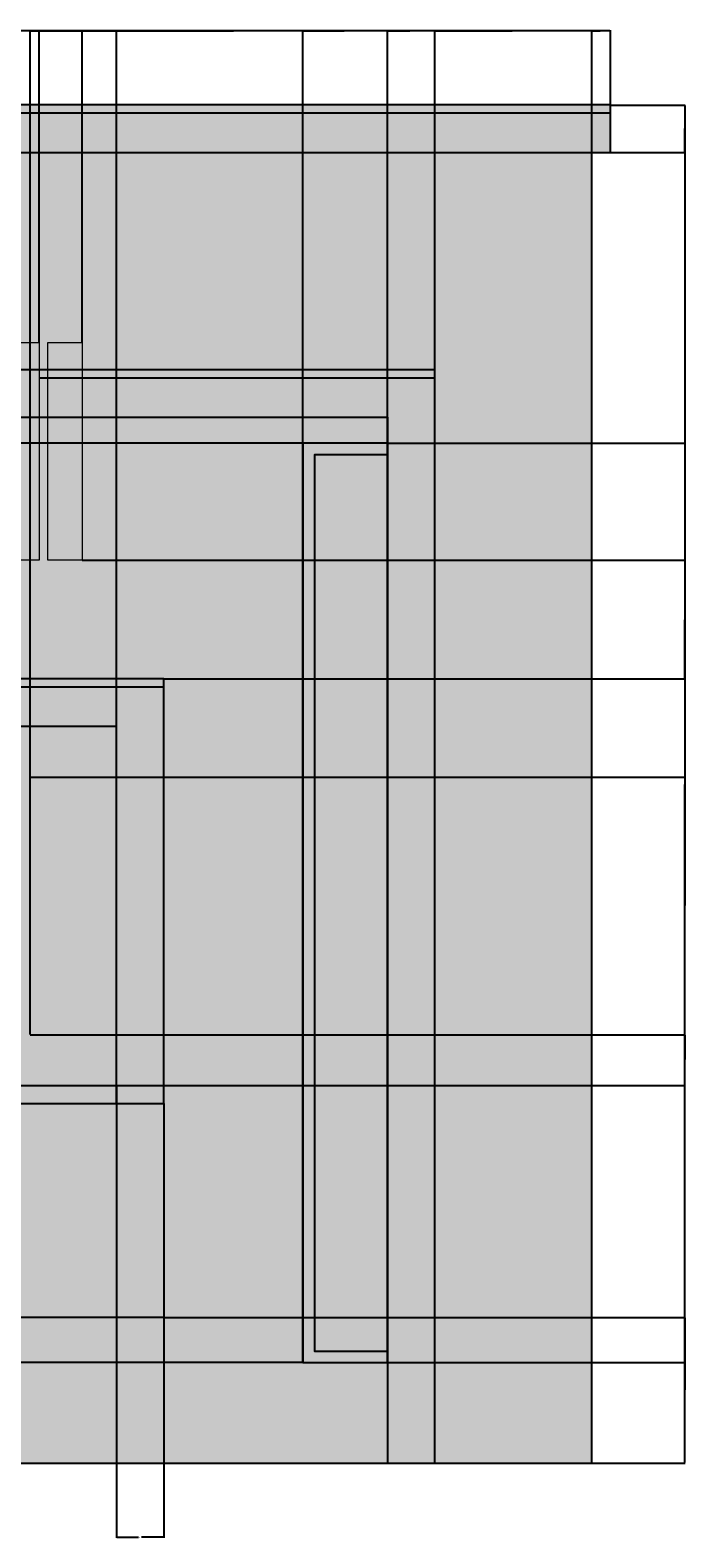
# Model space of a CAD drawing. Units: feet. Extents: x 2926 to 4178, y 965 to 1469.
# Tile 6 of 9: x 3245 to 3464, y 965 to 1469. Entities that reach past the tile are written whole.
import ezdxf

# ---------------------------------------------------------------- set-up
doc = ezdxf.new("R2010")
doc.units = ezdxf.units.FT
for name, color, linetype, lineweight in [('A-ANNO-DIMS', 2, 'Continuous', 18), ('A-ELEV', 7, 'Continuous', 25), ('A-ELEV-DETL', 8, 'Continuous', 18), ('A-ELEV-PATT', 9, 'Continuous', 13)]:
    doc.layers.add(name, color=color, linetype=linetype, lineweight=lineweight)
doc.styles.get("Standard").update_dxf_attribs({"font": 'arial.ttf'})
doc.dimstyles.get("Standard").update_dxf_attribs({"dimtxt": 0.18, "dimasz": 0.18, "dimexe": 0.18, "dimexo": 0.0625, "dimgap": 0.09, "dimtad": 0, "dimtih": 1, "dimtoh": 1, "dimdec": 1, "dimzin": 0, "dimdsep": 46, "dimlunit": 3, "dimtxsty": 'Standard', "dimcen": 0.09, "dimadec": 0, "dimazin": 0, "dimtfac": 1, "dimtdec": 1, "dimtofl": 0, "dimtmove": 0, "dimatfit": 3, "dimfxl": 1, "dimtolj": 1, "dimtzin": 0, "dimarcsym": 0})

# ---------------------------------------------------------------- blocks, each defined once
blk = doc.blocks.new('FACADE-FIN')
blk.add_lwpolyline([(0, 72.66), (11.46, 72.66), (11.46, 0), (0, 0)], close=True)
blk.add_lwpolyline([(0, 72.66), (11.46, 72.66), (11.46, 0), (0, 0)], close=True)
blk = doc.blocks.new('*D10')
at = {"layer": 'A-ANNO-DIMS', "color": 0, "lineweight": -2, "transparency": 16777216}
for p, q in [((2952.4, 1298.4), (2952.4, 1468.62)), ((2952.58, 1468.44), (3195.09, 1468.44)), ((3438.39, 1468.44), (3195.88, 1468.44)), ((3438.57, 1443.71), (3438.57, 1468.62))]:
    blk.add_line(p, q, dxfattribs=at)
at = {"layer": 'A-ANNO-DIMS', "color": 0, "transparency": 16777216}
for points in [[(2952.58, 1468.47), (2952.58, 1468.41), (2952.4, 1468.44)], [(3438.39, 1468.47), (3438.39, 1468.41), (3438.57, 1468.44)]]:
    blk.add_solid(points, dxfattribs=at)
at = {"layer": 'Defpoints', "color": 0, "transparency": 16777216}
for p in [(3438.57, 1468.44), (3438.57, 1443.64), (2952.4, 1298.33)]:
    blk.add_point(p, dxfattribs=at)
at = {"layer": 'A-ANNO-DIMS', "color": 0, "transparency": 16777216, "insert": (3195.49, 1468.44), "char_height": 0.18, "attachment_point": 5}
blk.add_mtext('\\A1;486.2', dxfattribs=at)
blk = doc.blocks.new('*D11')
at = {"layer": 'A-ANNO-DIMS', "color": 0, "lineweight": -2, "transparency": 16777216}
for p, q in [((3438.63, 1443.64), (3463.55, 1443.64)), ((3463.37, 1443.46), (3463.37, 1217.17)), ((3463.37, 990.5), (3463.37, 1216.8)), ((3432.46, 990.32), (3463.55, 990.32))]:
    blk.add_line(p, q, dxfattribs=at)
at = {"layer": 'A-ANNO-DIMS', "color": 0, "transparency": 16777216}
for points in [[(3463.34, 1443.46), (3463.4, 1443.46), (3463.37, 1443.64)], [(3463.34, 990.5), (3463.4, 990.5), (3463.37, 990.32)]]:
    blk.add_solid(points, dxfattribs=at)
at = {"layer": 'Defpoints', "color": 0, "transparency": 16777216}
for p in [(3438.57, 1443.64), (3463.37, 1443.64), (3432.4, 990.32)]:
    blk.add_point(p, dxfattribs=at)
at = {"layer": 'A-ANNO-DIMS', "color": 0, "transparency": 16777216, "insert": (3463.37, 1216.98), "char_height": 0.18, "attachment_point": 5}
blk.add_mtext('\\A1;453.3', dxfattribs=at)
blk = doc.blocks.new('*D12')
at = {"layer": 'A-ANNO-DIMS', "color": 0, "lineweight": -2, "transparency": 16777216}
for p, q in [((3335.85, 1023.86), (2926.57, 1023.86)), ((2926.75, 1023.68), (2926.75, 1007.27)), ((2926.75, 990.5), (2926.75, 1006.91)), ((2952.34, 990.32), (2926.57, 990.32))]:
    blk.add_line(p, q, dxfattribs=at)
at = {"layer": 'A-ANNO-DIMS', "color": 0, "transparency": 16777216}
for points in [[(2926.72, 1023.68), (2926.78, 1023.68), (2926.75, 1023.86)], [(2926.72, 990.5), (2926.78, 990.5), (2926.75, 990.32)]]:
    blk.add_solid(points, dxfattribs=at)
at = {"layer": 'Defpoints', "color": 0, "transparency": 16777216}
for p in [(2926.75, 1023.86), (3335.91, 1023.86), (2952.4, 990.32)]:
    blk.add_point(p, dxfattribs=at)
at = {"layer": 'A-ANNO-DIMS', "color": 0, "transparency": 16777216, "insert": (2926.75, 1007.09), "char_height": 0.18, "attachment_point": 5}
blk.add_mtext('\\A1;33.53', dxfattribs=at)
blk = doc.blocks.new('*D13')
at = {"layer": 'A-ANNO-DIMS', "color": 0, "lineweight": -2, "transparency": 16777216}
for p, q in [((3068.25, 1049.98), (2926.57, 1049.98)), ((2926.75, 1049.8), (2926.75, 1037.1)), ((2926.75, 1024.04), (2926.75, 1036.74)), ((3335.85, 1023.86), (2926.57, 1023.86))]:
    blk.add_line(p, q, dxfattribs=at)
at = {"layer": 'A-ANNO-DIMS', "color": 0, "transparency": 16777216}
for points in [[(2926.72, 1049.8), (2926.78, 1049.8), (2926.75, 1049.98)], [(2926.72, 1024.04), (2926.78, 1024.04), (2926.75, 1023.86)]]:
    blk.add_solid(points, dxfattribs=at)
at = {"layer": 'Defpoints', "color": 0, "transparency": 16777216}
for p in [(2926.75, 1049.98), (3068.31, 1049.98), (3335.91, 1023.86)]:
    blk.add_point(p, dxfattribs=at)
at = {"layer": 'A-ANNO-DIMS', "color": 0, "transparency": 16777216, "insert": (2926.75, 1036.92), "char_height": 0.18, "attachment_point": 5}
blk.add_mtext('\\A1;26.13', dxfattribs=at)
blk = doc.blocks.new('*D19')
at = {"layer": 'A-ANNO-DIMS', "color": 0, "lineweight": -2, "transparency": 16777216}
for p, q in [((3335.85, 1330.74), (2926.57, 1330.74)), ((2926.75, 1330.56), (2926.75, 1314.5)), ((2926.75, 1298.08), (2926.75, 1314.14)), ((2952.34, 1297.9), (2926.57, 1297.9))]:
    blk.add_line(p, q, dxfattribs=at)
at = {"layer": 'A-ANNO-DIMS', "color": 0, "transparency": 16777216}
for points in [[(2926.72, 1330.56), (2926.78, 1330.56), (2926.75, 1330.74)], [(2926.72, 1298.08), (2926.78, 1298.08), (2926.75, 1297.9)]]:
    blk.add_solid(points, dxfattribs=at)
at = {"layer": 'Defpoints', "color": 0, "transparency": 16777216}
for p in [(2926.75, 1330.74), (3335.91, 1330.74), (2952.4, 1297.9)]:
    blk.add_point(p, dxfattribs=at)
at = {"layer": 'A-ANNO-DIMS', "color": 0, "transparency": 16777216, "insert": (2926.75, 1314.32), "char_height": 0.18, "attachment_point": 5}
blk.add_mtext('\\A1;32.85', dxfattribs=at)
blk = doc.blocks.new('*D20')
at = {"layer": 'A-ANNO-DIMS', "color": 0, "lineweight": -2, "transparency": 16777216}
for p, q in [((3042.86, 1355.28), (2926.57, 1355.28)), ((2926.75, 1355.1), (2926.75, 1343.19)), ((2926.75, 1330.92), (2926.75, 1342.83)), ((3335.85, 1330.74), (2926.57, 1330.74))]:
    blk.add_line(p, q, dxfattribs=at)
at = {"layer": 'A-ANNO-DIMS', "color": 0, "transparency": 16777216}
for points in [[(2926.72, 1355.1), (2926.78, 1355.1), (2926.75, 1355.28)], [(2926.72, 1330.92), (2926.78, 1330.92), (2926.75, 1330.74)]]:
    blk.add_solid(points, dxfattribs=at)
at = {"layer": 'Defpoints', "color": 0, "transparency": 16777216}
for p in [(2926.75, 1355.28), (3042.92, 1355.28), (3335.91, 1330.74)]:
    blk.add_point(p, dxfattribs=at)
at = {"layer": 'A-ANNO-DIMS', "color": 0, "transparency": 16777216, "insert": (2926.75, 1343.01), "char_height": 0.18, "attachment_point": 5}
blk.add_mtext('\\A1;24.533', dxfattribs=at)
blk = doc.blocks.new('*D25')
at = {"layer": 'A-ANNO-DIMS', "color": 0, "lineweight": -2, "transparency": 16777216}
for p, q in [((3198.64, 1133.35), (3198.64, 1468.62)), ((3198.82, 1468.44), (3221.33, 1468.44)), ((3244.64, 1468.44), (3222.13, 1468.44)), ((3244.82, 1133.35), (3244.82, 1468.62))]:
    blk.add_line(p, q, dxfattribs=at)
at = {"layer": 'A-ANNO-DIMS', "color": 0, "transparency": 16777216}
for points in [[(3198.82, 1468.47), (3198.82, 1468.41), (3198.64, 1468.44)], [(3244.64, 1468.47), (3244.64, 1468.41), (3244.82, 1468.44)]]:
    blk.add_solid(points, dxfattribs=at)
at = {"layer": 'Defpoints', "color": 0, "transparency": 16777216}
for p in [(3244.82, 1468.44), (3198.64, 1133.29), (3244.82, 1133.29)]:
    blk.add_point(p, dxfattribs=at)
at = {"layer": 'A-ANNO-DIMS', "color": 0, "transparency": 16777216, "insert": (3221.73, 1468.44), "char_height": 0.18, "attachment_point": 5}
blk.add_mtext('\\A1;46.18', dxfattribs=at)
blk = doc.blocks.new('*D26')
at = {"layer": 'A-ANNO-DIMS', "color": 0, "lineweight": -2, "transparency": 16777216}
for p, q in [((3244.82, 1133.35), (3244.82, 1468.62)), ((3245, 1468.44), (3290.06, 1468.44)), ((3335.73, 1468.44), (3290.67, 1468.44)), ((3335.91, 1023.92), (3335.91, 1468.62))]:
    blk.add_line(p, q, dxfattribs=at)
at = {"layer": 'A-ANNO-DIMS', "color": 0, "transparency": 16777216}
for points in [[(3245, 1468.47), (3245, 1468.41), (3244.82, 1468.44)], [(3335.73, 1468.47), (3335.73, 1468.41), (3335.91, 1468.44)]]:
    blk.add_solid(points, dxfattribs=at)
at = {"layer": 'Defpoints', "color": 0, "transparency": 16777216}
for p in [(3335.91, 1468.44), (3244.82, 1133.29), (3335.91, 1023.86)]:
    blk.add_point(p, dxfattribs=at)
at = {"layer": 'A-ANNO-DIMS', "color": 0, "transparency": 16777216, "insert": (3290.37, 1468.44), "char_height": 0.18, "attachment_point": 5}
blk.add_mtext('\\A1;91.1', dxfattribs=at)
blk = doc.blocks.new('*D27')
at = {"layer": 'A-ANNO-DIMS', "color": 0, "lineweight": -2, "transparency": 16777216}
for p, q in [((3335.91, 1023.92), (3335.91, 1468.62)), ((3336.09, 1468.44), (3349.69, 1468.44)), ((3363.94, 1468.44), (3350.34, 1468.44)), ((3364.12, 1023.92), (3364.12, 1468.62))]:
    blk.add_line(p, q, dxfattribs=at)
at = {"layer": 'A-ANNO-DIMS', "color": 0, "transparency": 16777216}
for points in [[(3336.09, 1468.47), (3336.09, 1468.41), (3335.91, 1468.44)], [(3363.94, 1468.47), (3363.94, 1468.41), (3364.12, 1468.44)]]:
    blk.add_solid(points, dxfattribs=at)
at = {"layer": 'Defpoints', "color": 0, "transparency": 16777216}
for p in [(3364.12, 1468.44), (3335.91, 1023.86), (3364.12, 1023.86)]:
    blk.add_point(p, dxfattribs=at)
at = {"layer": 'A-ANNO-DIMS', "color": 0, "transparency": 16777216, "insert": (3350.02, 1468.44), "char_height": 0.18, "attachment_point": 5}
blk.add_mtext('\\A1;28.2', dxfattribs=at)
blk = doc.blocks.new('*D28')
at = {"layer": 'A-ANNO-DIMS', "color": 0, "lineweight": -2, "transparency": 16777216}
for p, q in [((3244.88, 1219.22), (3463.55, 1219.22)), ((3463.37, 1219.04), (3463.37, 1176.44)), ((3463.37, 1133.47), (3463.37, 1176.07)), ((3244.88, 1133.29), (3463.55, 1133.29))]:
    blk.add_line(p, q, dxfattribs=at)
at = {"layer": 'A-ANNO-DIMS', "color": 0, "transparency": 16777216}
for points in [[(3463.34, 1219.04), (3463.4, 1219.04), (3463.37, 1219.22)], [(3463.34, 1133.47), (3463.4, 1133.47), (3463.37, 1133.29)]]:
    blk.add_solid(points, dxfattribs=at)
at = {"layer": 'Defpoints', "color": 0, "transparency": 16777216}
for p in [(3244.82, 1219.22), (3463.37, 1219.22), (3244.82, 1133.29)]:
    blk.add_point(p, dxfattribs=at)
at = {"layer": 'A-ANNO-DIMS', "color": 0, "transparency": 16777216, "insert": (3463.37, 1176.25), "char_height": 0.18, "attachment_point": 5}
blk.add_mtext('\\A1;85.93', dxfattribs=at)
blk = doc.blocks.new('*D35')
at = {"layer": 'A-ANNO-DIMS', "color": 0, "lineweight": -2, "transparency": 16777216}
for p, q in [((3247.87, 1364.46), (3247.87, 1468.62)), ((3248.05, 1468.44), (3254.56, 1468.44)), ((3261.98, 1468.44), (3255.47, 1468.44)), ((3262.16, 1364.46), (3262.16, 1468.62))]:
    blk.add_line(p, q, dxfattribs=at)
at = {"layer": 'A-ANNO-DIMS', "color": 0, "transparency": 16777216}
for points in [[(3248.05, 1468.47), (3248.05, 1468.41), (3247.87, 1468.44)], [(3261.98, 1468.47), (3261.98, 1468.41), (3262.16, 1468.44)]]:
    blk.add_solid(points, dxfattribs=at)
at = {"layer": 'Defpoints', "color": 0, "transparency": 16777216}
for p in [(3262.16, 1468.44), (3247.87, 1364.4), (3262.16, 1364.4)]:
    blk.add_point(p, dxfattribs=at)
at = {"layer": 'A-ANNO-DIMS', "color": 0, "transparency": 16777216, "insert": (3255.02, 1468.44), "char_height": 0.18, "attachment_point": 5}
blk.add_mtext('\\A1;14.298', dxfattribs=at)
blk = doc.blocks.new('*D36')
at = {"layer": 'A-ANNO-DIMS', "color": 0, "lineweight": -2, "transparency": 16777216}
for p, q in [((3262.16, 1364.46), (3262.16, 1468.62)), ((3262.34, 1468.44), (3312.68, 1468.44)), ((3363.94, 1468.44), (3313.6, 1468.44)), ((3364.12, 1339.53), (3364.12, 1468.62))]:
    blk.add_line(p, q, dxfattribs=at)
at = {"layer": 'A-ANNO-DIMS', "color": 0, "transparency": 16777216}
for points in [[(3262.34, 1468.47), (3262.34, 1468.41), (3262.16, 1468.44)], [(3363.94, 1468.47), (3363.94, 1468.41), (3364.12, 1468.44)]]:
    blk.add_solid(points, dxfattribs=at)
at = {"layer": 'Defpoints', "color": 0, "transparency": 16777216}
for p in [(3364.12, 1468.44), (3262.16, 1364.4), (3364.12, 1339.46)]:
    blk.add_point(p, dxfattribs=at)
at = {"layer": 'A-ANNO-DIMS', "color": 0, "transparency": 16777216, "insert": (3313.14, 1468.44), "char_height": 0.18, "attachment_point": 5}
blk.add_mtext('\\A1;101.95', dxfattribs=at)
blk = doc.blocks.new('*D37')
at = {"layer": 'A-ANNO-DIMS', "color": 0, "lineweight": -2, "transparency": 16777216}
for p, q in [((3364.12, 1339.53), (3364.12, 1468.62)), ((3364.3, 1468.44), (3371.57, 1468.44)), ((3379.75, 1468.44), (3372.48, 1468.44)), ((3379.93, 1355.34), (3379.93, 1468.62))]:
    blk.add_line(p, q, dxfattribs=at)
at = {"layer": 'A-ANNO-DIMS', "color": 0, "transparency": 16777216}
for points in [[(3364.3, 1468.47), (3364.3, 1468.41), (3364.12, 1468.44)], [(3379.75, 1468.47), (3379.75, 1468.41), (3379.93, 1468.44)]]:
    blk.add_solid(points, dxfattribs=at)
at = {"layer": 'Defpoints', "color": 0, "transparency": 16777216}
for p in [(3379.93, 1468.44), (3379.93, 1355.28), (3364.12, 1339.46)]:
    blk.add_point(p, dxfattribs=at)
at = {"layer": 'A-ANNO-DIMS', "color": 0, "transparency": 16777216, "insert": (3372.02, 1468.44), "char_height": 0.18, "attachment_point": 5}
blk.add_mtext('\\A1;15.814', dxfattribs=at)
blk = doc.blocks.new('*D38')
at = {"layer": 'A-ANNO-DIMS', "color": 0, "lineweight": -2, "transparency": 16777216}
for p, q in [((3379.93, 1355.34), (3379.93, 1468.62)), ((3380.11, 1468.44), (3405.77, 1468.44)), ((3432.22, 1468.44), (3406.56, 1468.44)), ((3432.4, 1427.89), (3432.4, 1468.62))]:
    blk.add_line(p, q, dxfattribs=at)
at = {"layer": 'A-ANNO-DIMS', "color": 0, "transparency": 16777216}
for points in [[(3380.11, 1468.47), (3380.11, 1468.41), (3379.93, 1468.44)], [(3432.22, 1468.47), (3432.22, 1468.41), (3432.4, 1468.44)]]:
    blk.add_solid(points, dxfattribs=at)
at = {"layer": 'Defpoints', "color": 0, "transparency": 16777216}
for p in [(3432.4, 1468.44), (3432.4, 1427.83), (3379.93, 1355.28)]:
    blk.add_point(p, dxfattribs=at)
at = {"layer": 'A-ANNO-DIMS', "color": 0, "transparency": 16777216, "insert": (3406.17, 1468.44), "char_height": 0.18, "attachment_point": 5}
blk.add_mtext('\\A1;52.47', dxfattribs=at)
blk = doc.blocks.new('*D39')
at = {"layer": 'A-ANNO-DIMS', "color": 0, "lineweight": -2, "transparency": 16777216}
for p, q in [((3432.4, 1427.89), (3432.4, 1468.62)), ((3432.58, 1468.44), (3435.09, 1468.44)), ((3438.39, 1468.44), (3435.88, 1468.44)), ((3438.57, 1443.71), (3438.57, 1468.62))]:
    blk.add_line(p, q, dxfattribs=at)
at = {"layer": 'A-ANNO-DIMS', "color": 0, "transparency": 16777216}
for points in [[(3432.58, 1468.47), (3432.58, 1468.41), (3432.4, 1468.44)], [(3438.39, 1468.47), (3438.39, 1468.41), (3438.57, 1468.44)]]:
    blk.add_solid(points, dxfattribs=at)
at = {"layer": 'Defpoints', "color": 0, "transparency": 16777216}
for p in [(3438.57, 1468.44), (3438.57, 1443.64), (3432.4, 1427.83)]:
    blk.add_point(p, dxfattribs=at)
at = {"layer": 'A-ANNO-DIMS', "color": 0, "transparency": 16777216, "insert": (3435.49, 1468.44), "char_height": 0.18, "attachment_point": 5}
blk.add_mtext('\\A1;6.169', dxfattribs=at)
blk = doc.blocks.new('*D40')
at = {"layer": 'A-ANNO-DIMS', "color": 0, "lineweight": -2, "transparency": 16777216}
for p, q in [((3438.63, 1443.64), (3463.55, 1443.64)), ((3463.37, 1443.46), (3463.37, 1435.92)), ((3463.37, 1428.01), (3463.37, 1435.56)), ((3438.63, 1427.83), (3463.55, 1427.83))]:
    blk.add_line(p, q, dxfattribs=at)
at = {"layer": 'A-ANNO-DIMS', "color": 0, "transparency": 16777216}
for points in [[(3463.34, 1443.46), (3463.4, 1443.46), (3463.37, 1443.64)], [(3463.34, 1428.01), (3463.4, 1428.01), (3463.37, 1427.83)]]:
    blk.add_solid(points, dxfattribs=at)
at = {"layer": 'Defpoints', "color": 0, "transparency": 16777216}
for p in [(3438.57, 1443.64), (3463.37, 1443.64), (3438.57, 1427.83)]:
    blk.add_point(p, dxfattribs=at)
at = {"layer": 'A-ANNO-DIMS', "color": 0, "transparency": 16777216, "insert": (3463.37, 1435.74), "char_height": 0.18, "attachment_point": 5}
blk.add_mtext('\\A1;15.814', dxfattribs=at)
blk = doc.blocks.new('*D43')
at = {"layer": 'A-ANNO-DIMS', "color": 0, "lineweight": -2, "transparency": 16777216}
for p, q in [((3262.23, 1291.73), (3463.55, 1291.73)), ((3463.37, 1291.55), (3463.37, 1272.12)), ((3463.37, 1252.32), (3463.37, 1271.75)), ((3289.48, 1252.14), (3463.55, 1252.14))]:
    blk.add_line(p, q, dxfattribs=at)
at = {"layer": 'A-ANNO-DIMS', "color": 0, "transparency": 16777216}
for points in [[(3463.34, 1291.55), (3463.4, 1291.55), (3463.37, 1291.73)], [(3463.34, 1252.32), (3463.4, 1252.32), (3463.37, 1252.14)]]:
    blk.add_solid(points, dxfattribs=at)
at = {"layer": 'Defpoints', "color": 0, "transparency": 16777216}
for p in [(3262.16, 1291.73), (3463.37, 1291.73), (3289.41, 1252.14)]:
    blk.add_point(p, dxfattribs=at)
at = {"layer": 'A-ANNO-DIMS', "color": 0, "transparency": 16777216, "insert": (3463.37, 1271.94), "char_height": 0.18, "attachment_point": 5}
blk.add_mtext('\\A1;39.596', dxfattribs=at)
blk = doc.blocks.new('*D44')
at = {"layer": 'A-ANNO-DIMS', "color": 0, "lineweight": -2, "transparency": 16777216}
for p, q in [((3364.18, 1330.74), (3463.55, 1330.74)), ((3463.37, 1330.56), (3463.37, 1177.48)), ((3463.37, 1024.04), (3463.37, 1177.12)), ((3364.18, 1023.86), (3463.55, 1023.86))]:
    blk.add_line(p, q, dxfattribs=at)
at = {"layer": 'A-ANNO-DIMS', "color": 0, "transparency": 16777216}
for points in [[(3463.34, 1330.56), (3463.4, 1330.56), (3463.37, 1330.74)], [(3463.34, 1024.04), (3463.4, 1024.04), (3463.37, 1023.86)]]:
    blk.add_solid(points, dxfattribs=at)
at = {"layer": 'Defpoints', "color": 0, "transparency": 16777216}
for p in [(3364.12, 1330.74), (3463.37, 1330.74), (3364.12, 1023.86)]:
    blk.add_point(p, dxfattribs=at)
at = {"layer": 'A-ANNO-DIMS', "color": 0, "transparency": 16777216, "insert": (3463.37, 1177.3), "char_height": 0.18, "attachment_point": 5}
blk.add_mtext('\\A1;306.9', dxfattribs=at)
blk = doc.blocks.new('*D62')
at = {"layer": 'A-ANNO-DIMS', "color": 0, "lineweight": -2, "transparency": 16777216}
for p, q in [((3273.6, 1116.26), (3273.6, 965.34)), ((3289.41, 1110.26), (3289.41, 965.34)), ((3273.78, 965.52), (3281.05, 965.52)), ((3289.23, 965.52), (3281.96, 965.52))]:
    blk.add_line(p, q, dxfattribs=at)
at = {"layer": 'A-ANNO-DIMS', "color": 0, "transparency": 16777216}
for points in [[(3273.78, 965.55), (3273.78, 965.49), (3273.6, 965.52)], [(3289.23, 965.55), (3289.23, 965.49), (3289.41, 965.52)]]:
    blk.add_solid(points, dxfattribs=at)
at = {"layer": 'Defpoints', "color": 0, "transparency": 16777216}
for p in [(3273.6, 1116.32), (3289.41, 1110.32), (3289.41, 965.52)]:
    blk.add_point(p, dxfattribs=at)
at = {"layer": 'A-ANNO-DIMS', "color": 0, "transparency": 16777216, "insert": (3281.51, 965.52), "char_height": 0.18, "attachment_point": 5}
blk.add_mtext('\\A1;15.814', dxfattribs=at)
blk = doc.blocks.new('*D63')
at = {"layer": 'A-ANNO-DIMS', "color": 0, "lineweight": -2, "transparency": 16777216}
for p, q in [((3244.82, 1219.28), (3244.82, 1468.62)), ((3245, 1468.44), (3258.81, 1468.44)), ((3273.42, 1468.44), (3259.6, 1468.44)), ((3273.6, 1236.39), (3273.6, 1468.62))]:
    blk.add_line(p, q, dxfattribs=at)
at = {"layer": 'A-ANNO-DIMS', "color": 0, "transparency": 16777216}
for points in [[(3245, 1468.47), (3245, 1468.41), (3244.82, 1468.44)], [(3273.42, 1468.47), (3273.42, 1468.41), (3273.6, 1468.44)]]:
    blk.add_solid(points, dxfattribs=at)
at = {"layer": 'Defpoints', "color": 0, "transparency": 16777216}
for p in [(3273.6, 1468.44), (3273.6, 1236.32), (3244.82, 1219.22)]:
    blk.add_point(p, dxfattribs=at)
at = {"layer": 'A-ANNO-DIMS', "color": 0, "transparency": 16777216, "insert": (3259.21, 1468.44), "char_height": 0.18, "attachment_point": 5}
blk.add_mtext('\\A1;28.78', dxfattribs=at)
blk = doc.blocks.new('*D64')
at = {"layer": 'A-ANNO-DIMS', "color": 0, "lineweight": -2, "transparency": 16777216}
for p, q in [((3244.88, 1133.29), (3463.55, 1133.29)), ((3463.37, 1133.11), (3463.37, 1124.99)), ((3463.37, 1116.5), (3463.37, 1124.62)), ((3273.66, 1116.32), (3463.55, 1116.32))]:
    blk.add_line(p, q, dxfattribs=at)
at = {"layer": 'A-ANNO-DIMS', "color": 0, "transparency": 16777216}
for points in [[(3463.34, 1133.11), (3463.4, 1133.11), (3463.37, 1133.29)], [(3463.34, 1116.5), (3463.4, 1116.5), (3463.37, 1116.32)]]:
    blk.add_solid(points, dxfattribs=at)
at = {"layer": 'Defpoints', "color": 0, "transparency": 16777216}
for p in [(3244.82, 1133.29), (3463.37, 1133.29), (3273.6, 1116.32)]:
    blk.add_point(p, dxfattribs=at)
at = {"layer": 'A-ANNO-DIMS', "color": 0, "transparency": 16777216, "insert": (3463.37, 1124.81), "char_height": 0.18, "attachment_point": 5}
blk.add_mtext('\\A1;16.963', dxfattribs=at)
blk = doc.blocks.new('*D65')
at = {"layer": 'A-ANNO-DIMS', "color": 0, "lineweight": -2, "transparency": 16777216}
for p, q in [((3289.48, 1038.92), (3463.55, 1038.92)), ((3463.37, 1038.74), (3463.37, 1014.8)), ((3463.37, 990.5), (3463.37, 1014.44)), ((3364.18, 990.32), (3463.55, 990.32))]:
    blk.add_line(p, q, dxfattribs=at)
at = {"layer": 'A-ANNO-DIMS', "color": 0, "transparency": 16777216}
for points in [[(3463.34, 1038.74), (3463.4, 1038.74), (3463.37, 1038.92)], [(3463.34, 990.5), (3463.4, 990.5), (3463.37, 990.32)]]:
    blk.add_solid(points, dxfattribs=at)
at = {"layer": 'Defpoints', "color": 0, "transparency": 16777216}
for p in [(3289.41, 1038.92), (3364.12, 990.32), (3463.37, 990.32)]:
    blk.add_point(p, dxfattribs=at)
at = {"layer": 'A-ANNO-DIMS', "color": 0, "transparency": 16777216, "insert": (3463.37, 1014.62), "char_height": 0.18, "attachment_point": 5}
blk.add_mtext('\\A1;48.6', dxfattribs=at)

msp = doc.modelspace()

# ---------------------------------------------------------------- hatches: boundary and pattern name
at = {"layer": 'A-ELEV-PATT'}
h = msp.add_hatch(color=256, dxfattribs=at)
h.dxf.hatch_style = 1
h.paths.add_polyline_path([(2968.9852, 1110.3246), (2958.1139, 1110.3246), (2958.1139, 1060.462), (2968.9852, 1060.462)])
h.paths.add_polyline_path([(3174.217, 1126.1389), (2952.4018, 1126.1389), (2952.4018, 1110.3246), (3174.217, 1110.3246), (3273.5987, 1110.3246), (3273.5987, 1116.3246), (3174.217, 1116.3246)], flags=17)
h.paths.add_polyline_path([(3289.413, 1252.1389), (2952.4018, 1252.1389), (2952.4018, 1236.3246), (3273.5987, 1236.3246), (3273.5987, 1110.3246), (3289.413, 1110.3246)])
h.paths.add_polyline_path([(3221.3497, 1355.2778), (3042.9199, 1355.2778), (3042.9199, 1339.4635), (3221.3497, 1339.4635)])
h.paths.add_polyline_path([(3379.9311, 1355.2778), (3262.1646, 1355.2778), (3262.1646, 1339.4635), (3364.1168, 1339.4635), (3364.1168, 990.3246), (3379.9311, 990.3246)])
h.paths.add_polyline_path([(3364.1168, 1330.7444), (3335.9143, 1330.7444), (3335.9143, 1023.8561), (3364.1168, 1023.8561), (3364.1168, 1027.6935), (3339.7517, 1027.6935), (3339.7517, 1326.907), (3364.1168, 1326.907)], flags=17)
h.paths.add_polyline_path([(3438.5707, 1443.6445), (3153.6951, 1443.6445), (3153.6951, 1427.8302), (3438.5707, 1427.8302)])
h.paths.add_polyline_path([(3174.217, 1427.8302), (3153.6951, 1427.8302), (3174.217, 1356.4366)])
h.paths.add_polyline_path([(3174.217, 1339.4635), (3042.9199, 1339.4635), (3070.6809, 1317.1829), (3174.217, 1317.1829)])
h.paths.add_polyline_path([(3244.819, 1219.2195), (3198.6415, 1219.2195), (3198.6415, 1133.2879), (3244.819, 1133.2879)], flags=17)
h = msp.add_hatch(color=256, dxfattribs=at)
h.dxf.hatch_style = 1
h.paths.add_polyline_path([(3006.649, 1296.2176), (2952.4018, 1296.2176), (2952.4018, 1252.1389), (3006.649, 1252.1389)])
h.paths.add_polyline_path([(3084.0314, 1226.8042), (3008.2802, 1226.8042), (3008.2802, 1171.8963), (3084.0314, 1171.8963)])
h.paths.add_polyline_path([(3004.9276, 1228.4641), (2995.6704, 1228.4641), (2995.6704, 1171.8963), (3004.9276, 1171.8963)])
h.paths.add_polyline_path([(3174.217, 1236.3246), (3084.0314, 1236.3246), (3084.0314, 1171.8963), (3124.7575, 1171.8963), (3124.7575, 1207.1083), (3154.7729, 1207.1083), (3154.7729, 1171.8963), (3174.217, 1171.8963)])
h.paths.add_polyline_path([(3273.5987, 1236.3246), (3174.217, 1236.3246), (3174.217, 1171.8963), (3174.217, 1126.1389), (3174.217, 1116.3246), (3273.5987, 1116.3246)], flags=16)
h.paths.add_polyline_path([(3198.6415, 1219.2195), (3244.819, 1219.2195), (3244.819, 1133.2879), (3198.6415, 1133.2879)], flags=0)
h.paths.add_polyline_path([(3432.4018, 1427.8302), (3174.217, 1427.8302), (3174.217, 1356.4366), (3174.5501, 1355.2778), (3221.3497, 1355.2778), (3221.3497, 1364.3965), (3232.8063, 1364.3965), (3232.8063, 1355.2778), (3236.4098, 1355.2778), (3236.4098, 1364.3965), (3247.8663, 1364.3965), (3247.8663, 1355.2778), (3250.7081, 1355.2778), (3250.7081, 1364.3965), (3262.1646, 1364.3965), (3262.1646, 1355.2778), (3379.9311, 1355.2778), (3379.9311, 990.3246), (3432.4018, 990.3246)])
h.paths.add_polyline_path([(3068.3128, 1092.0439), (3130.6886, 1092.0439), (3130.6886, 1049.9841), (3146.6469, 1049.9841), (3146.6469, 1057.7915), (3145.2184, 1058.2122), (3145.2184, 1060.462), (3168.644, 1060.462), (3174.217, 1058.8204), (3174.217, 1110.3246), (3004.9276, 1110.3246), (3004.9276, 1049.9841), (3068.3128, 1049.9841)])
h.paths.add_polyline_path([(3174.217, 1056.3197), (3152.4954, 1056.3197), (3152.4954, 990.3246), (3174.217, 990.3246)])
h.paths.add_polyline_path([(2974.1234, 1056.3197), (2952.4018, 1056.3197), (2952.4018, 990.3246), (2974.1234, 990.3246)])
h.paths.add_polyline_path([(3004.9276, 1110.3246), (2995.6704, 1110.3246), (2995.6704, 1049.9841), (3004.9276, 1049.9841)])
h = msp.add_hatch(color=256, dxfattribs=at)
h.dxf.hatch_style = 1
h.paths.add_polyline_path([(3262.1646, 1339.4635), (3250.7081, 1339.4635), (3250.7081, 1291.7348), (3262.1646, 1291.7348)])
h.paths.add_polyline_path([(3262.1646, 1355.2778), (3250.7081, 1355.2778), (3250.7081, 1339.4635), (3262.1646, 1339.4635)])
h.paths.add_polyline_path([(3262.1646, 1364.3965), (3250.7081, 1364.3965), (3250.7081, 1355.2778), (3262.1646, 1355.2778)])
h.paths.add_polyline_path([(3247.8663, 1364.3965), (3236.4098, 1364.3965), (3236.4098, 1355.2778), (3247.8663, 1355.2778)])
h.paths.add_polyline_path([(3247.8663, 1355.2778), (3236.4098, 1355.2778), (3236.4098, 1339.4635), (3247.8663, 1339.4635)])
h.paths.add_polyline_path([(3247.8663, 1339.4635), (3236.4098, 1339.4635), (3236.4098, 1291.7348), (3247.8663, 1291.7348)])
h.paths.add_polyline_path([(3232.8063, 1339.4635), (3221.3497, 1339.4635), (3221.3497, 1291.7348), (3232.8063, 1291.7348)])
h.paths.add_polyline_path([(3232.8063, 1355.2778), (3221.3497, 1355.2778), (3221.3497, 1339.4635), (3232.8063, 1339.4635)])
h.paths.add_polyline_path([(3232.8063, 1364.3965), (3221.3497, 1364.3965), (3221.3497, 1355.2778), (3232.8063, 1355.2778)])
h = msp.add_hatch(color=256, dxfattribs=at)
h.dxf.hatch_style = 1
h.paths.add_polyline_path([(3335.9143, 1330.7444), (3364.1168, 1330.7444), (3364.1168, 1339.4635), (3262.1646, 1339.4635), (3262.1646, 1291.7348), (3250.7081, 1291.7348), (3250.7081, 1339.4635), (3247.8663, 1339.4635), (3247.8663, 1291.7348), (3236.4098, 1291.7348), (3236.4098, 1339.4635), (3232.8063, 1339.4635), (3232.8063, 1291.7348), (3221.3497, 1291.7348), (3221.3497, 1339.4635), (3174.217, 1339.4635), (3174.217, 1252.1389), (3289.413, 1252.1389), (3289.413, 1236.3246), (3289.413, 1110.3246), (3289.413, 1038.9216), (3174.217, 1038.9216), (3174.217, 990.3246), (3364.1168, 990.3246), (3364.1168, 1023.8561), (3335.9143, 1023.8561)])
h.paths.add_polyline_path([(3236.4098, 1355.2778), (3232.8063, 1355.2778), (3232.8063, 1339.4635), (3236.4098, 1339.4635)])
h.paths.add_polyline_path([(3250.7081, 1355.2778), (3247.8663, 1355.2778), (3247.8663, 1339.4635), (3250.7081, 1339.4635)])
h = msp.add_hatch(color=256, dxfattribs=at)
h.dxf.hatch_style = 1
h.paths.add_polyline_path([(3174.217, 1297.8963), (3172.3488, 1297.8963), (3006.649, 1297.8963), (3006.649, 1296.2176), (3087.9974, 1296.2176), (3087.9974, 1252.1389), (3089.8656, 1252.1389), (3089.8656, 1296.2176), (3172.3488, 1296.2176), (3172.3488, 1252.1389), (3174.217, 1252.1389)])
h.paths.add_polyline_path([(3102.4583, 1170.2176), (3172.3488, 1170.2176), (3172.3488, 1126.1389), (3174.217, 1126.1389), (3174.217, 1171.8963), (3172.3488, 1171.8963), (2952.4018, 1171.8963), (2952.4018, 1170.2176), (2952.4018, 1126.1389), (2954.27, 1126.1389), (2954.27, 1170.2176), (3100.5901, 1170.2176), (3100.5901, 1126.1389), (3102.4583, 1126.1389)])
h.paths.add_polyline_path([(3130.6886, 1092.0439), (3068.3128, 1092.0439), (3068.3128, 1049.9841), (3130.6886, 1049.9841)])
h.paths.add_polyline_path([(3099.0016, 1090.4638), (3099.0016, 1051.5643), (3069.893, 1051.5643), (3069.893, 1090.4638)], flags=16)
h.paths.add_polyline_path([(3099.9998, 1090.4638), (3129.1085, 1090.4638), (3129.1085, 1051.5643), (3099.9998, 1051.5643)], flags=16)
h.paths.add_polyline_path([(3067.2712, 1049.9841), (3060.102, 1049.9841), (3060.102, 990.3246), (3067.2712, 990.3246)])
h.paths.add_polyline_path([(3339.7517, 1326.907), (3364.1168, 1326.907), (3364.1168, 1330.7444), (3335.9143, 1330.7444), (3335.9143, 1023.8561), (3364.1168, 1023.8561), (3364.1168, 1027.6935), (3339.7517, 1027.6935)])
h.paths.add_polyline_path([(3154.7729, 1207.1083), (3124.7575, 1207.1083), (3124.7575, 1171.8963), (3126.8684, 1171.8963), (3126.8684, 1204.9974), (3152.6619, 1204.9974), (3152.6619, 1171.8963), (3154.7729, 1171.8963)])
h = msp.add_hatch(color=256, dxfattribs=at)
h.dxf.hatch_style = 1
h.paths.add_polyline_path([(3070.6809, 1296.2176), (3006.649, 1296.2176), (3006.649, 1252.1389), (3070.6809, 1252.1389)])
h.paths.add_polyline_path([(3087.9974, 1296.2176), (3070.6809, 1296.2176), (3070.6809, 1252.1389), (3087.9974, 1252.1389)])
h.paths.add_polyline_path([(3172.3488, 1296.2176), (3089.8656, 1296.2176), (3089.8656, 1252.1389), (3172.3488, 1252.1389)])
h.paths.add_polyline_path([(3152.6619, 1170.2176), (3126.8684, 1170.2176), (3126.8684, 1128.2498), (3152.6619, 1128.2498)], flags=17)
h.paths.add_polyline_path([(3152.6619, 1204.9974), (3126.8684, 1204.9974), (3126.8684, 1171.8963), (3152.6619, 1171.8963)])
h.paths.add_polyline_path([(3172.3488, 1170.2176), (3154.7729, 1170.2176), (3154.7729, 1126.1389), (3172.3488, 1126.1389)])
h.paths.add_polyline_path([(3154.7729, 1170.2176), (3152.6619, 1170.2176), (3152.6619, 1128.2498), (3126.8684, 1128.2498), (3126.8684, 1170.2176), (3124.7575, 1170.2176), (3124.7575, 1126.1389), (3154.7729, 1126.1389)])
h.paths.add_polyline_path([(3124.7575, 1170.2176), (3102.4583, 1170.2176), (3102.4583, 1126.1389), (3124.7575, 1126.1389)])
h.paths.add_polyline_path([(3100.5901, 1170.2176), (3084.0314, 1170.2176), (3084.0314, 1126.1389), (3100.5901, 1126.1389)])
h.paths.add_polyline_path([(3084.0314, 1170.2176), (3008.2802, 1170.2176), (3008.2802, 1126.1389), (3084.0314, 1126.1389)])
h.paths.add_polyline_path([(2995.6704, 1170.2176), (2971.1978, 1170.2176), (2971.1978, 1126.1389), (2995.6704, 1126.1389)])
h.paths.add_polyline_path([(3004.9276, 1170.2176), (2995.6704, 1170.2176), (2995.6704, 1126.1389), (3004.9276, 1126.1389)])
h.paths.add_polyline_path([(3364.1168, 1326.907), (3339.7517, 1326.907), (3339.7517, 1027.6935), (3364.1168, 1027.6935)])
h.paths.add_polyline_path([(3099.0016, 1090.4638), (3069.893, 1090.4638), (3069.893, 1051.5643), (3099.0016, 1051.5643)])
h.paths.add_polyline_path([(3129.1085, 1090.4638), (3099.9998, 1090.4638), (3099.9998, 1051.5643), (3129.1085, 1051.5643)])
h.paths.add_polyline_path([(2968.9852, 1170.2176), (2958.1139, 1170.2176), (2958.1139, 1126.1389), (2968.9852, 1126.1389)])
h.paths.add_polyline_path([(2958.1139, 1170.2176), (2954.27, 1170.2176), (2954.27, 1126.1389), (2958.1139, 1126.1389)])
h.paths.add_polyline_path([(2971.1978, 1170.2176), (2968.9852, 1170.2176), (2968.9852, 1126.1389), (2971.1978, 1126.1389)])
h = msp.add_hatch(color=256, dxfattribs=at)
h.dxf.hatch_style = 1
h.paths.add_polyline_path([(3289.413, 1110.3246), (3174.217, 1110.3246), (3174.217, 1058.8204), (3175.069, 1058.5694), (3175.069, 1056.3197), (3174.217, 1056.3197), (3174.217, 1038.9216), (3289.413, 1038.9216)])

# ---------------------------------------------------------------- linework, layer by layer
at = {"layer": 'A-ELEV'}
for p, q in [((3153.6951, 1440.9727), (3438.5707, 1440.9727)), ((3438.5707, 1427.8302), (3438.5707, 1443.6445)), ((3438.5707, 1427.8302), (3438.5707, 1443.6445)), ((3432.4018, 990.3246), (3432.4018, 1427.8302)), ((3432.4018, 990.3246), (3432.4018, 1427.8302)), ((3247.8663, 1352.606), (3379.9311, 1352.606)), ((3364.1168, 1339.4635), (3364.1168, 990.3246)), ((3364.1168, 1339.4635), (3364.1168, 990.3246)), ((2952.4018, 1249.4671), (3289.413, 1249.4671)), ((3289.413, 1110.3246), (3289.413, 1252.1389)), ((3289.413, 1110.3246), (3289.413, 1252.1389)), ((2952.4018, 1236.3246), (3273.5987, 1236.3246)), ((2952.4018, 1236.3246), (3273.5987, 1236.3246)), ((3273.5987, 1110.3246), (3273.5987, 1236.3246)), ((3273.5987, 1110.3246), (3273.5987, 1236.3246)), ((3174.217, 1116.3246), (3273.5987, 1116.3246)), ((3174.217, 1116.3246), (3273.5987, 1116.3246)), ((2952.4018, 1110.3246), (3289.413, 1110.3246)), ((2952.4018, 1110.3246), (3289.413, 1110.3246)), ((3289.413, 1110.3246), (3289.413, 1038.9216)), ((3289.413, 1110.3246), (3289.413, 1038.9216)), ((3289.413, 1038.9216), (3174.217, 1038.9216)), ((3289.413, 1038.9216), (3174.217, 1038.9216)), ((2952.4018, 990.3246), (3432.4018, 990.3246)), ((2952.4018, 990.3246), (3432.4018, 990.3246))]:
    msp.add_line(p, q, dxfattribs=at)
for points in [[(3438.5707, 1443.6445), (3153.6951, 1443.6445), (3153.6951, 1427.8302), (3438.5707, 1427.8302)], [(3438.5707, 1443.6445), (3153.6951, 1443.6445), (3153.6951, 1427.8302), (3438.5707, 1427.8302)], [(3379.9311, 990.3246), (3379.9311, 1355.2778), (3042.9199, 1355.2778), (3042.9199, 1339.4635), (3364.1168, 1339.4635)], [(3250.7081, 1355.2778), (3247.8663, 1355.2778)], [(3379.9311, 990.3246), (3379.9311, 1355.2778), (3262.1646, 1355.2778)], [(3247.8663, 1339.4635), (3250.7081, 1339.4635)], [(3262.1646, 1339.4635), (3364.1168, 1339.4635)], [(3364.1168, 1326.907), (3339.7517, 1326.907), (3339.7517, 1027.6935), (3364.1168, 1027.6935)], [(3364.1168, 1326.907), (3339.7517, 1326.907), (3339.7517, 1027.6935), (3364.1168, 1027.6935)], [(3289.413, 1236.3246), (3289.413, 1252.1389), (2952.4018, 1252.1389), (2952.4018, 1236.3246), (3273.5987, 1236.3246)], [(3289.413, 1236.3246), (3289.413, 1252.1389), (2952.4018, 1252.1389), (2952.4018, 1236.3246), (3273.5987, 1236.3246)]]:
    msp.add_lwpolyline(points, dxfattribs=at)
msp.add_lwpolyline([(3364.1168, 1330.7444), (3335.9143, 1330.7444), (3335.9143, 1023.8561), (3364.1168, 1023.8561)], close=True, dxfattribs=at)
msp.add_lwpolyline([(3364.1168, 1330.7444), (3335.9143, 1330.7444), (3335.9143, 1023.8561), (3364.1168, 1023.8561)], close=True, dxfattribs=at)

# ---------------------------------------------------------------- block references
at = {"layer": 'A-ELEV-DETL'}
for p in [(3236.4101, 1291.735), (3250.7084, 1291.735)]:
    msp.add_blockref('FACADE-FIN', p, dxfattribs=at)

# ---------------------------------------------------------------- dimensions: what is measured, and where the dimension line sits
at = {"layer": 'A-ANNO-DIMS'}
for base, p1, p2, override, picture, middle in [((3438.5707, 1468.4445), (2952.4018, 1298.3338), (3438.5707, 1443.6445), {"dimdec": 1, "dimlfac": 1, "dimrnd": 0, "dimzin": 0, "dimdsep": 46, "dimlunit": 2}, '*D10', (3195.4862, 1468.4445)), ((3244.819, 1468.4445), (3198.6415, 1133.2879), (3244.819, 1133.2879), {"dimdec": 2, "dimlfac": 1, "dimrnd": 0, "dimzin": 0, "dimdsep": 46, "dimlunit": 2}, '*D25', (3221.7303, 1468.4445)), ((3335.9143, 1468.4445), (3244.819, 1133.2879), (3335.9143, 1023.8561), {"dimdec": 1, "dimlfac": 1, "dimrnd": 0, "dimzin": 0, "dimdsep": 46, "dimlunit": 2}, '*D26', (3290.3667, 1468.4445)), ((3273.5987, 1468.4445), (3244.819, 1219.2195), (3273.5987, 1236.3246), {"dimdec": 2, "dimlfac": 1, "dimrnd": 0, "dimzin": 0, "dimdsep": 46, "dimlunit": 2}, '*D63', (3259.2089, 1468.4445)), ((3262.1646, 1468.4445), (3247.8663, 1364.3965), (3262.1646, 1364.3965), {"dimdec": 3, "dimlfac": 1, "dimrnd": 0, "dimzin": 0, "dimdsep": 46, "dimlunit": 2}, '*D35', (3255.0155, 1468.4445)), ((3364.1168, 1468.4445), (3262.1646, 1364.3965), (3364.1168, 1339.4635), {"dimdec": 2, "dimlfac": 1, "dimrnd": 0, "dimzin": 0, "dimdsep": 46, "dimlunit": 2}, '*D36', (3313.1407, 1468.4445)), ((3364.1168, 1468.4445), (3335.9143, 1023.8561), (3364.1168, 1023.8561), {"dimdec": 1, "dimlfac": 1, "dimrnd": 0, "dimzin": 0, "dimdsep": 46, "dimlunit": 2}, '*D27', (3350.0156, 1468.4445)), ((3379.9311, 1468.4445), (3364.1168, 1339.4635), (3379.9311, 1355.2778), {"dimdec": 3, "dimlfac": 1, "dimrnd": 0, "dimzin": 0, "dimdsep": 46, "dimlunit": 2}, '*D37', (3372.024, 1468.4445)), ((3432.4018, 1468.4445), (3379.9311, 1355.2778), (3432.4018, 1427.8302), {"dimdec": 2, "dimlfac": 1, "dimrnd": 0, "dimzin": 0, "dimdsep": 46, "dimlunit": 2}, '*D38', (3406.1665, 1468.4445)), ((3438.5707, 1468.4445), (3432.4018, 1427.8302), (3438.5707, 1443.6445), {"dimdec": 3, "dimlfac": 1, "dimrnd": 0, "dimzin": 0, "dimdsep": 46, "dimlunit": 2}, '*D39', (3435.4862, 1468.4445)), ((3289.413, 965.5246), (3273.5987, 1116.3246), (3289.413, 1110.3246), {"dimdec": 3, "dimlfac": 1, "dimrnd": 0, "dimzin": 0, "dimdsep": 46, "dimlunit": 2}, '*D62', (3281.5059, 965.5246))]:
    dim = msp.add_linear_dim(base=base, p1=p1, p2=p2, dimstyle='Standard', override=override, dxfattribs=at)
    dim.commit()
    dim.dimension.update_dxf_attribs({"geometry": picture, "text_midpoint": middle})
for base, p1, p2, override, picture, middle in [((3463.3707, 1443.6445), (3432.4018, 990.3246), (3438.5707, 1443.6445), {"dimdec": 1, "dimlfac": 1, "dimrnd": 0, "dimzin": 0, "dimdsep": 46, "dimlunit": 2}, '*D11', (3463.3707, 1216.9845)), ((3463.3707, 1443.6445), (3438.5707, 1427.8302), (3438.5707, 1443.6445), {"dimdec": 3, "dimlfac": 1, "dimrnd": 0, "dimzin": 0, "dimdsep": 46, "dimlunit": 2}, '*D40', (3463.3707, 1435.7374)), ((2926.7498, 1355.2778), (3335.9143, 1330.7444), (3042.9199, 1355.2778), {"dimdec": 3, "dimlfac": 1, "dimrnd": 0, "dimzin": 0, "dimdsep": 46, "dimlunit": 2}, '*D20', (2926.7498, 1343.0111)), ((2926.7498, 1330.7444), (2952.4018, 1297.8963), (3335.9143, 1330.7444), {"dimdec": 2, "dimlfac": 1, "dimrnd": 0, "dimzin": 0, "dimdsep": 46, "dimlunit": 2}, '*D19', (2926.7498, 1314.3203)), ((3463.3707, 1330.7444), (3364.1168, 1023.8561), (3364.1168, 1330.7444), {"dimdec": 1, "dimlfac": 1, "dimrnd": 0, "dimzin": 0, "dimdsep": 46, "dimlunit": 2}, '*D44', (3463.3707, 1177.3002)), ((3463.3707, 1291.7348), (3289.413, 1252.1389), (3262.1646, 1291.7348), {"dimdec": 3, "dimlfac": 1, "dimrnd": 0, "dimzin": 0, "dimdsep": 46, "dimlunit": 2}, '*D43', (3463.3707, 1271.9368)), ((3463.3707, 1219.2195), (3244.819, 1133.2879), (3244.819, 1219.2195), {"dimdec": 2, "dimlfac": 1, "dimrnd": 0, "dimzin": 0, "dimdsep": 46, "dimlunit": 2}, '*D28', (3463.3707, 1176.2537)), ((3463.3707, 1133.2879), (3273.5987, 1116.3246), (3244.819, 1133.2879), {"dimdec": 3, "dimlfac": 1, "dimrnd": 0, "dimzin": 0, "dimdsep": 46, "dimlunit": 2}, '*D64', (3463.3707, 1124.8062)), ((2926.7498, 1049.9841), (3335.9143, 1023.8561), (3068.3128, 1049.9841), {"dimdec": 2, "dimlfac": 1, "dimrnd": 0, "dimzin": 0, "dimdsep": 46, "dimlunit": 2}, '*D13', (2926.7498, 1036.9201)), ((3463.3707, 990.3246), (3289.413, 1038.9216), (3364.1168, 990.3246), {"dimdec": 1, "dimlfac": 1, "dimrnd": 0, "dimzin": 0, "dimdsep": 46, "dimlunit": 2}, '*D65', (3463.3707, 1014.6231)), ((2926.7498, 1023.8561), (2952.4018, 990.3246), (3335.9143, 1023.8561), {"dimdec": 2, "dimlfac": 1, "dimrnd": 0, "dimzin": 0, "dimdsep": 46, "dimlunit": 2}, '*D12', (2926.7498, 1007.0903))]:
    dim = msp.add_linear_dim(base=base, p1=p1, p2=p2, angle=90, dimstyle='Standard', override=override, dxfattribs=at)
    dim.commit()
    dim.dimension.update_dxf_attribs({"geometry": picture, "text_midpoint": middle})

doc.saveas('drawing.dxf')
